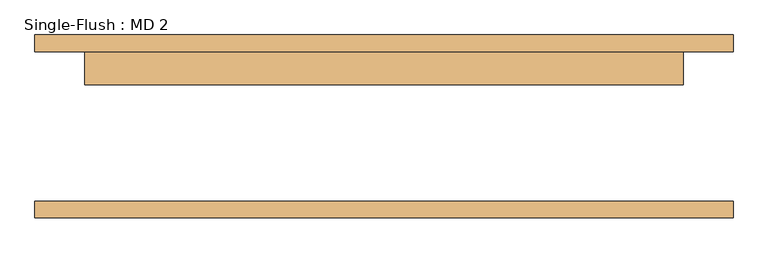
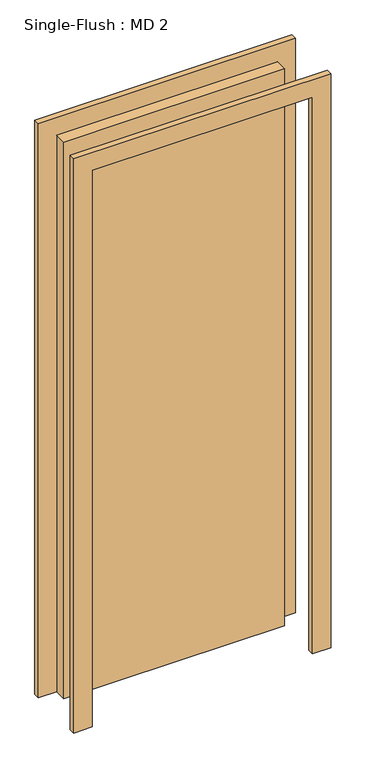
"""IFC4 building model written with IfcOpenShell, lengths in millimetres: door geometry, Single-Flush : MD 2."""

from ifc_helpers import new_model, si_unit, frame, origin, origin_with_axes, place, context, project, spatial, polyline, outline, extrude, source, transform, mapped, element, save


def single_flush_md_2_408f135a(model_context):
    return source(origin(), model_context, "Body", "SweptSolid", [
        extrude(outline(polyline([(2514.6, -533.4), (0.0, -533.4), (0.0, -457.2), (2438.4, -457.2), (2438.4, 457.2), (0.0, 457.2), (0.0, 533.4), (2514.6, 533.4), (2514.6, -533.4)])), frame((0.0, 114.3, 0.0), z_axis=(0.0, 1.0, 0.0), x_axis=(0.0, 0.0, 1.0)), (0.0, 0.0, 1.0), 25.4),
        extrude(outline(polyline([(2514.6, 533.4), (2514.6, -533.4), (0.0, -533.4), (0.0, -457.2), (2438.4, -457.2), (2438.4, 457.2), (0.0, 457.2), (0.0, 533.4), (2514.6, 533.4)])), frame((0.0, -139.7, 0.0), z_axis=(0.0, 1.0, 0.0), x_axis=(0.0, 0.0, 1.0)), (0.0, 0.0, 1.0), 25.4),
        extrude(outline(polyline([(457.2, 63.5), (-457.2, 63.5), (-457.2, 114.3), (457.2, 114.3), (457.2, 63.5)])), origin_with_axes(), (0.0, 0.0, 1.0), 2438.4),
    ])


if __name__ == "__main__":
    model = new_model("IFC4")
    model_context = context("Model", 3, world=origin())
    ifc_project = project(units=[si_unit("LENGTHUNIT", "METRE", prefix="MILLI")], contexts=[model_context])
    site = spatial("IfcSite", under=ifc_project)
    building = spatial("IfcBuilding", under=site)
    placement = place(None, origin())
    single_flush_md_2_shape = single_flush_md_2_408f135a(model_context)
    element("IfcDoor", 1, ObjectType="Single-Flush : MD 2", at=placement, inside=building, context=model_context, shape_type="MappedRepresentation", body=[
        mapped(single_flush_md_2_shape, transform((0.0, 0.0, 0.0), x_axis=(1.0, 0.0, 0.0), y_axis=(0.0, 1.0, 0.0), z_axis=(0.0, 0.0, 1.0))),
    ])
    save(model, "model.ifc")

# Revit data of these elements
# Type "Single-Flush : MD 2"
#   Type Mark = "11"
#   Construction Type Id = "MDOOR"
#   Assembly Code = "C1020"
#   Analytic Construction = "Metal"
#   Thickness = 0' - 2"
#   Heat Transfer Coefficient (U) = 0.651978 BTU/(h·ft²·°F)
#   Height = 8' - 0"
#   Trim Projection Ext = 0' - 1"
#   Trim Projection Int = 0' - 1"
#   Trim Width = 0' - 3"
#   Width = 3' - 0"
#   Define Thermal Properties by = 1
#   Door Material = Door - Panel
#   Frame Material = Door - Frame
#   Visual Light Transmittance = 0
#   Solar Heat Gain Coefficient = 0
#   Function = (empty or 0)
#   Wall Closure = (empty or 0)
# Element 1 (IfcDoor, "Single-Flush : MD 2")
#   Materials on its faces: "Door - Frame", "Door - Panel"
# Materials
#   "Door - Panel": class "Wood", colour RGB 210 159 95, transparency 0, Cost = 0
#   "Door - Frame": colour RGB 118 70 51, transparency 0, Cost = 0
